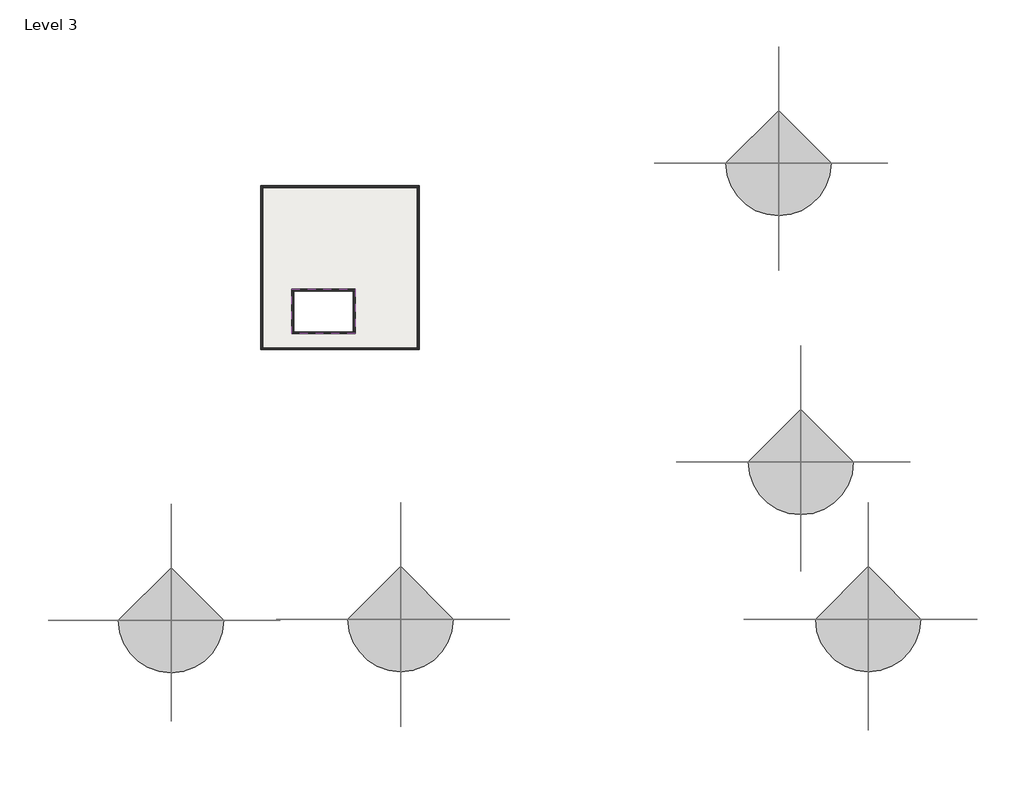
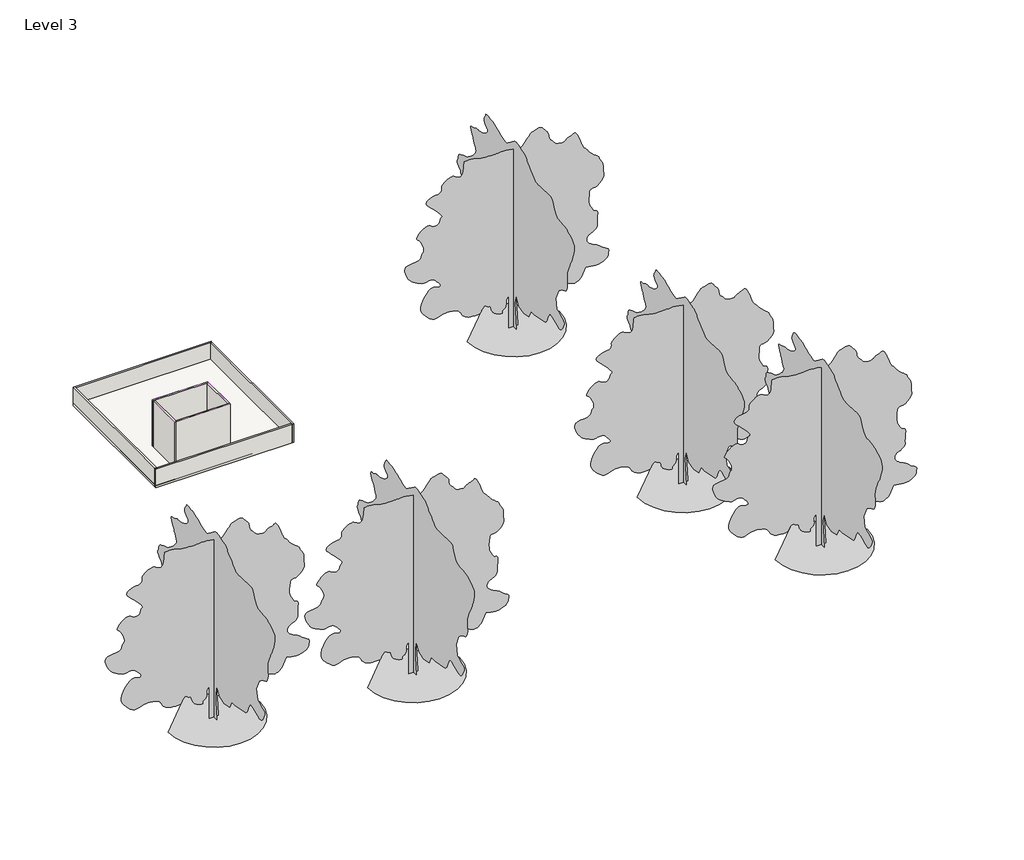
# One storey: 8 walls, 5 geographic elements, 1 covering, 1 slab.
"""IFC4 building model written with IfcOpenShell, lengths in millimetres."""

from ifc_helpers import new_model, si_unit, frame, origin, place, context, project, spatial, polyline, outline, extrude, faceted_brep, transform, mapped, element, save
from components import m_rpc_tree_deciduous_scarlet_oak_12_5_meters_78a4568a

model = new_model("IFC4")

# Units and contexts
model_context = context("Model", 3, world=origin())
ifc_project = project(units=[si_unit("LENGTHUNIT", "METRE", prefix="MILLI")], contexts=[model_context])

# Site, building, storey
site = spatial("IfcSite", under=ifc_project)
building = spatial("IfcBuilding", under=site)
storey = spatial("IfcBuildingStorey", under=building, Name="Level 3", Elevation=6400.8)

# Covering
placement = place(None, origin())
element("IfcCovering", 1, ObjectType="Plain", at=placement, inside=storey, context=model_context, shape_type="SweptSolid", body=[
    extrude(outline(polyline([(-9970.9646777, -4404.6421603), (-9970.9646777, -1983.5421603), (-6531.1282945, -1983.5421603), (-6531.1282945, -4404.6421603), (-9970.9646777, -4404.6421603)])), frame((0.0, 0.0, 9601.2), z_axis=(0.0, 0.0, 1.0), x_axis=(1.0, 0.0, 0.0)), (0.0, 0.0, 1.0), 57.0),
])

# Geographic elements
m_rpc_tree_deciduous_scarlet_oak_12_5_meters_shape = m_rpc_tree_deciduous_scarlet_oak_12_5_meters_78a4568a(model_context)
element("IfcGeographicElement", 2, ObjectType="M_RPC Tree - Deciduous : Scarlet Oak - 12.5 Meters", at=placement, inside=storey, context=model_context, shape_type="MappedRepresentation", body=[
    mapped(m_rpc_tree_deciduous_scarlet_oak_12_5_meters_shape, transform((16445.6374905, 4860.5343745, 1034.8394056), x_axis=(1.0, 0.0, 0.0), y_axis=(0.0, 1.0, 0.0), z_axis=(0.0, 0.0, 1.0))),
])
element("IfcGeographicElement", 3, ObjectType="M_RPC Tree - Deciduous : Scarlet Oak - 12.5 Meters", at=placement, inside=storey, context=model_context, shape_type="MappedRepresentation", body=[
    mapped(m_rpc_tree_deciduous_scarlet_oak_12_5_meters_shape, transform((17653.3990587, -11368.7940322, 203.0988084), x_axis=(1.0, 0.0, 0.0), y_axis=(0.0, 1.0, 0.0), z_axis=(0.0, 0.0, 1.0))),
])
element("IfcGeographicElement", 4, ObjectType="M_RPC Tree - Deciduous : Scarlet Oak - 12.5 Meters", at=placement, inside=storey, context=model_context, shape_type="MappedRepresentation", body=[
    mapped(m_rpc_tree_deciduous_scarlet_oak_12_5_meters_shape, transform((-4066.3201453, -19903.1446672, 478.283371), x_axis=(1.0, 0.0, 0.0), y_axis=(0.0, 1.0, 0.0), z_axis=(0.0, 0.0, 1.0))),
])
element("IfcGeographicElement", 5, ObjectType="M_RPC Tree - Deciduous : Scarlet Oak - 12.5 Meters", at=placement, inside=storey, context=model_context, shape_type="MappedRepresentation", body=[
    mapped(m_rpc_tree_deciduous_scarlet_oak_12_5_meters_shape, transform((21310.7717055, -19903.2421603, 0.0), x_axis=(1.0, 0.0, 0.0), y_axis=(0.0, 1.0, 0.0), z_axis=(0.0, 0.0, 1.0))),
])
element("IfcGeographicElement", 6, ObjectType="M_RPC Tree - Deciduous : Scarlet Oak - 12.5 Meters", at=placement, inside=storey, context=model_context, shape_type="MappedRepresentation", body=[
    mapped(m_rpc_tree_deciduous_scarlet_oak_12_5_meters_shape, transform((-16521.5248182, -19965.8059564, 1940.0316245), x_axis=(1.0, 0.0, 0.0), y_axis=(0.0, 1.0, 0.0), z_axis=(0.0, 0.0, 1.0))),
])

# Slab
element("IfcSlab", 7, ObjectType="Generic 150mm", at=placement, inside=storey, context=model_context, shape_type="SweptSolid", body=[
    extrude(outline(polyline([(-3064.4329612, 3642.5578397), (-3064.4329612, -5272.8421603), (-11658.4282945, -5272.8421603), (-11658.4282945, 3642.5578397), (-3064.4329612, 3642.5578397)]), holes=[polyline([(-9869.3646777, -4303.0421603), (-6632.7282945, -4303.0421603), (-6632.7282945, -2085.1421603), (-9869.3646777, -2085.1421603), (-9869.3646777, -4303.0421603)])]), frame((0.0, 0.0, 6403.2), z_axis=(0.0, 0.0, 1.0), x_axis=(1.0, 0.0, 0.0)), (0.0, 0.0, 1.0), 150.0),
])

# Walls
element("IfcWall", 8, ObjectType="4\"", at=placement, inside=storey, context=model_context, shape_type="Brep", body=[
    faceted_brep([(-3073.2282945, 3642.5578397, 6400.8), (-11550.3644632, 3642.5578397, 6400.8), (-11550.3644632, 3642.5578397, 7620.0), (-3073.2282945, 3642.5578397, 7620.0), (-3073.2282945, 3540.9578397, 6400.8), (-3073.2282945, 3540.9578397, 7620.0), (-3174.8282945, 3540.9578397, 7620.0), (-11550.3644632, 3540.9578397, 7620.0), (-11550.3644632, 3540.9578397, 6400.8), (-3174.8282945, 3540.9578397, 6400.8)], [[[0, 1, 2, 3]], [[4, 5, 6, 7, 8, 9]], [[1, 0, 4, 9, 8]], [[3, 2, 7, 6, 5]], [[0, 3, 5, 4]], [[2, 1, 8, 7]]]),
])
element("IfcWall", 9, ObjectType="4\"", at=placement, inside=storey, context=model_context, shape_type="Brep", body=[
    faceted_brep([(-3073.2282945, -5272.8421603, 6400.8), (-3073.2282945, 3540.9578397, 6400.8), (-3073.2282945, 3540.9578397, 7620.0), (-3073.2282945, -5272.8421603, 7620.0), (-3174.8282945, -5272.8421603, 6400.8), (-3174.8282945, -5272.8421603, 7620.0), (-3174.8282945, -5171.2421603, 7620.0), (-3174.8282945, 3540.9578397, 7620.0), (-3174.8282945, 3540.9578397, 6400.8), (-3174.8282945, -5171.2421603, 6400.8)], [[[0, 1, 2, 3]], [[4, 5, 6, 7, 8, 9]], [[1, 0, 4, 9, 8]], [[3, 2, 7, 6, 5]], [[0, 3, 5, 4]], [[2, 1, 8, 7]]]),
])
element("IfcWall", 10, ObjectType="4\"", at=placement, inside=storey, context=model_context, shape_type="Brep", body=[
    faceted_brep([(-11651.9644632, -5272.8421603, 6400.8), (-3174.8282945, -5272.8421603, 6400.8), (-3174.8282945, -5272.8421603, 7620.0), (-11651.9644632, -5272.8421603, 7620.0), (-11651.9644632, -5171.2421603, 6400.8), (-11651.9644632, -5171.2421603, 7620.0), (-11550.3644632, -5171.2421603, 7620.0), (-3174.8282945, -5171.2421603, 7620.0), (-3174.8282945, -5171.2421603, 6400.8), (-11550.3644632, -5171.2421603, 6400.8)], [[[0, 1, 2, 3]], [[4, 5, 6, 7, 8, 9]], [[1, 0, 4, 9, 8]], [[3, 2, 7, 6, 5]], [[0, 3, 5, 4]], [[2, 1, 8, 7]]]),
])
element("IfcWall", 11, ObjectType="4\"", at=placement, inside=storey, context=model_context, shape_type="Brep", body=[
    faceted_brep([(-11651.9644632, 3642.5578397, 6400.8), (-11651.9644632, -5171.2421603, 6400.8), (-11651.9644632, -5171.2421603, 7620.0), (-11651.9644632, 3642.5578397, 7620.0), (-11550.3644632, 3642.5578397, 6400.8), (-11550.3644632, 3642.5578397, 7620.0), (-11550.3644632, 3540.9578397, 7620.0), (-11550.3644632, -5171.2421603, 7620.0), (-11550.3644632, -5171.2421603, 6400.8), (-11550.3644632, 3540.9578397, 6400.8)], [[[0, 1, 2, 3]], [[4, 5, 6, 7, 8, 9]], [[1, 0, 4, 9, 8]], [[3, 2, 7, 6, 5]], [[0, 3, 5, 4]], [[2, 1, 8, 7]]]),
])
element("IfcWall", 12, ObjectType="4\"", at=placement, inside=storey, context=model_context, shape_type="Brep", body=[
    faceted_brep([(-6531.1282945, -1983.5421603, 6400.8), (-9970.9646777, -1983.5421603, 6400.8), (-9970.9646777, -1983.5421603, 9601.2), (-6531.1282945, -1983.5421603, 9601.2), (-6531.1282945, -2085.1421603, 6400.8), (-6531.1282945, -2085.1421603, 9601.2), (-6632.7282945, -2085.1421603, 9601.2), (-9869.3646777, -2085.1421603, 9601.2), (-9970.9646777, -2085.1421603, 9601.2), (-9970.9646777, -2085.1421603, 6400.8), (-9869.3646777, -2085.1421603, 6400.8), (-6632.7282945, -2085.1421603, 6400.8)], [[[0, 1, 2, 3]], [[4, 5, 6, 7, 8, 9, 10, 11]], [[1, 0, 4, 11, 10, 9]], [[3, 2, 8, 7, 6, 5]], [[2, 1, 9, 8]], [[0, 3, 5, 4]]]),
])
element("IfcWall", 13, ObjectType="4\"", at=placement, inside=storey, context=model_context, shape_type="Brep", body=[
    faceted_brep([(-9970.9646777, -2085.1421603, 6400.8), (-9970.9646777, -4404.6421603, 6400.8), (-9970.9646777, -4404.6421603, 9601.2), (-9970.9646777, -2085.1421603, 9601.2), (-9869.3646777, -2085.1421603, 6400.8), (-9869.3646777, -2085.1421603, 9601.2), (-9869.3646777, -4303.0421603, 9601.2), (-9869.3646777, -4404.6421603, 9601.2), (-9869.3646777, -4404.6421603, 6400.8), (-9869.3646777, -4303.0421603, 6400.8)], [[[0, 1, 2, 3]], [[4, 5, 6, 7, 8, 9]], [[1, 0, 4, 9, 8]], [[3, 2, 7, 6, 5]], [[0, 3, 5, 4]], [[2, 1, 8, 7]]]),
])
element("IfcWall", 14, ObjectType="4\"", at=placement, inside=storey, context=model_context, shape_type="Brep", body=[
    faceted_brep([(-9869.3646777, -4404.6421603, 6400.8), (-6531.1282945, -4404.6421603, 6400.8), (-6531.1282945, -4404.6421603, 9601.2), (-9869.3646777, -4404.6421603, 9601.2), (-9869.3646777, -4303.0421603, 6400.8), (-9869.3646777, -4303.0421603, 9601.2), (-6632.7282945, -4303.0421603, 9601.2), (-6531.1282945, -4303.0421603, 9601.2), (-6531.1282945, -4303.0421603, 6400.8), (-6632.7282945, -4303.0421603, 6400.8)], [[[0, 1, 2, 3]], [[4, 5, 6, 7, 8, 9]], [[1, 0, 4, 9, 8]], [[3, 2, 7, 6, 5]], [[0, 3, 5, 4]], [[2, 1, 8, 7]]]),
])
element("IfcWall", 15, ObjectType="4\"", at=placement, inside=storey, context=model_context, shape_type="SweptSolid", body=[
    extrude(outline(polyline([(-6531.1282945, -2085.1421603), (-6531.1282945, -4303.0421603), (-6632.7282945, -4303.0421603), (-6632.7282945, -2085.1421603), (-6531.1282945, -2085.1421603)])), frame((0.0, 0.0, 6400.8), z_axis=(0.0, 0.0, 1.0), x_axis=(1.0, 0.0, 0.0)), (0.0, 0.0, 1.0), 3200.4),
])

save(model, "model.ifc")

# Revit data of these elements
# Type "Plain"
#   built-in parameter 1002203 = 1 (stored number, unit not read)
#   built-in parameter 1002202 = 1 (stored number, unit not read)
#   Layers, outside or top first: 0' - 1.77165" "Metal Stud Layer" (function 1); 0' - 0.47244" "Gypsum Wall Board" (function 1)
# Type "M_RPC Tree - Deciduous : Scarlet Oak - 12.5 Meters"
#   built-in parameter 1005198 = "{2, 15},{39, RPC-16-G0FB-J5PX-0LX6-U000-ST1L-LVER-AU},{1, 0},{1, 0},{2, 35},{1, 8},{5, Color},{1, 0},{1, 0},{3, 0.8},{3, 0.8},{3, 0.8},{1, 8},{7, BBoxMin},{1, 0},{1, 0},{1, 0},{1, 0},{1, 0},{1, 8},{7, BBoxMax},{1, 0},{1, 0},{1, 0},{1, 0},{1, 0},{2, 11},{9, RPCTypeId},{1, 0},{1, 0},{39, RPC-16-G0FB-J5PX-0LX6-U000-ST1L-LVER-AU},{1, 6},{14, RPCPlantHeight},{1, 0},{1, 0},{7, 41.0105},{2, 11},{7, keyword},{1, 0},{1, 0},{128, :Geometry:RPC:Scarlet_Oak:Quercus palustris:Occurs in southern Ontario at the east and west ends of Lake Erie; locally abundant.},{2, 11},{8, category},{1, 0},{1, 0},{16, :Trees [General]},{2, 11},{12, LocalizedUID},{1, 0},{1, 0},{11, Scarlet_Oak},{2, 14},{6, Height},{1, 0},{1, 0},{7, 41.0105},{1, 2},{16, Cast Reflections},{1, 0},{1, 0},{1, 0},{1, 2},{12, Cast Shadows},{1, 0},{1, 0},{1, 1},{1, 2},{9, Lock View},{1, 0},{1, 0},{1, 0},{1, 4},{5, ViewC},{1, 0},{1, 0},{1, 0},{2, 11},{20, AdvancedUIDefinition},{1, 0},{1, 0},{0, },{2, 11},{10, AssetLibID},{1, 0},{1, 0},{36, 4D3F6E72-3F99-4203-98E9-AF80B3C7A7A4},{2, 11},{10, BaseSchema},{1, 0},{1, 0},{9, RPCSchema},{2, 11},{12, ExchangeGUID},{1, 0},{1, 0},{0, },{1, 2},{6, Hidden},{1, 0},{1, 0},{1, 0},{1, 4},{11, RPCCategory},{1, 0},{1, 0},{1, 0},{2, 11},{8, RPCImage},{1, 0},{1, 0},{0, },{1, 4},{13, SchemaVersion},{1, 0},{1, 0},{1, 4},{2, 11},{12, UIDefinition},{1, 0},{1, 0},{0, },{2, 11},{6, UIName},{1, 0},{1, 0},{39, RPC-16-G0FB-J5PX-0LX6-U000-ST1L-LVER-AU},{2, 11},{11, VersionGUID},{1, 0},{1, 0},{9, RPCSchema},{2, 11},{9, assettype},{1, 0},{1, 0},{11, RPCGeometry},{2, 11},{11, description},{1, 0},{1, 0},{0, },{2, 11},{9, localname},{1, 0},{1, 0},{3, RPC},{2, 11},{9, localtype},{1, 0},{1, 0},{3, RPC},{1, 4},{8, revision},{1, 0},{1, 0},{1, 1},{2, 11},{9, thumbnail},{1, 0},{1, 0},{0, },{1, 4},{7, version},{1, 0},{1, 0},{1, 1},{1, 2},{20, RPC_Cast Reflections},{1, 0},{1, 0},{1, 1},{1, 2},{16, RPC_Cast Shadows},{1, 0},{1, 0},{1, 1},{1, 2},{13, RPC_Lock View},{1, 0},{1, 0},{1, 0},{1, 4},{9, RPC_ViewC},{1, 0},{1, 0},{1, 0},{21, assetlibrary_base.fbx},{1, 5},"
#   built-in parameter 1005195 = "RPC-16-G0FB-J5PX-0LX6-U000-ST1L-LVER-AU"
#   Type Comments = "Scarlet Oak"
#   Height = 41' - 0.12598"
#   Default Elevation = 0
# Type "Generic 150mm"
#   Function = 0
#   Layers, outside or top first: 0' - 5.90551" no material (function 1)
# Type "4\""
#   Layers, outside or top first: 0' - 4" no material (function 1)
# Element 1 (IfcCovering, "Plain")
#   Height Offset From Level = 10' - 6"
#   Phase Created = New Construction
#   Materials on its faces: "Gypsum Wall Board", "Concrete, Cast-in-Place, Gray"
# Elements 2, 3, 4, 5, 6 (IfcGeographicElement, "M_RPC Tree - Deciduous : Scarlet Oak - 12.5 Meters")
#   Phase Created = New Construction
# Element 7 (IfcSlab, "Generic 150mm")
#   Height Offset From Level = 0' - 6"
#   Phase Created = New Construction
#   Materials on its faces: "Default Floor", "OUTER WALL", "Concrete, Cast-in-Place, Gray"
# Elements 8, 9, 10, 11 (IfcWall, "4\"")
#   Top Offset = 0' - 0"
#   Base Offset = 0' - 0"
#   Unconnected Height = 4' - 0"
#   wall height = 4' - 0"
#   Phase Created = New Construction
#   Base Constraint = Level 3
#   Materials on its faces: "OUTER WALL", "Default Wall"
# Element 12 (IfcWall, "4\"")
#   Top Offset = 0' - 0"
#   Base Offset = 0' - 0"
#   Unconnected Height = 10' - 6"
#   wall height = 10' - 6"
#   Phase Created = New Construction
#   Base Constraint = Level 3
#   Materials on its faces: "OUTER WALL", "Default Wall"
# Elements 13, 14, 15 (IfcWall, "4\"")
#   Top Offset = 0' - 0"
#   Base Offset = 0' - 0"
#   Unconnected Height = 10' - 6"
#   wall height = 10' - 6"
#   Phase Created = New Construction
#   Base Constraint = Level 3
#   Materials on its faces: "Default Wall", "OUTER WALL"
# Materials
#   "Metal Stud Layer": class "Metal", colour RGB 127 127 127, transparency 0, Description = "Light gauge steel framing, thermal air layer", Cost = 0
#   "Gypsum Wall Board": class "Generic", colour RGB 249 249 249, transparency 0, Description = "Gypsum Wall Board", Cost = 0
#   "Concrete, Cast-in-Place, Gray": class "Concrete", colour RGB 192 192 192, transparency 0, Description = "Cast-in-place concrete", Cost = 0
#   "Default Floor": colour RGB 127 127 127, transparency 0, Cost = 0
#   "OUTER WALL": class "Generic", colour RGB 120 120 120, transparency 0, Cost = 0
#   "Default Wall": colour RGB 128 128 128, transparency 0, Cost = 0
